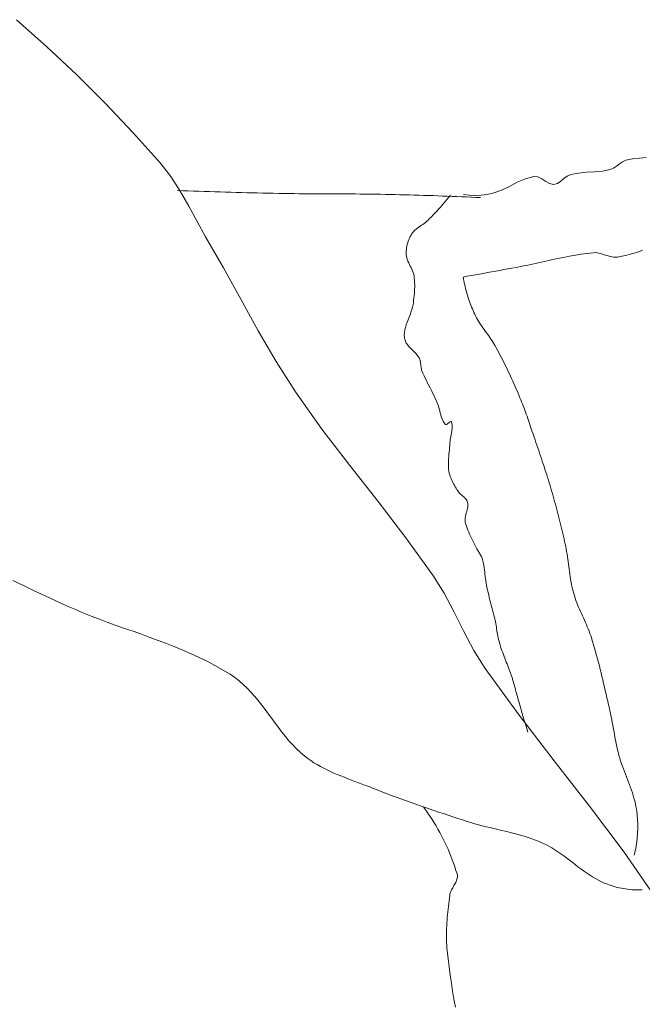
# Model space of a CAD drawing. Units: inches. Extents: x -36302355 to 648, y -221479757 to 75.
# Tile 19 of 37: x 555 to 572, y -501 to -474. Entities that reach past the tile are written whole.
import ezdxf

# ---------------------------------------------------------------- set-up
doc = ezdxf.new("R2010")
doc.units = ezdxf.units.IN
doc.header["$MEASUREMENT"] = 0
doc.layers.add('A-FURN', color=8, linetype='Continuous', lineweight=13)

# ---------------------------------------------------------------- blocks, each defined once
blk = doc.blocks.new('BED-DOUBLE')
for p, q in [((24.695, 63.097), (23.379, 62.192)), ((4.096, 62.613), (4.083, 62.806)), ((6.696, 62.587), (6.657, 62.702)), ((24.428, 62.63), (24.425, 62.688)), ((4.119, 62.421), (4.096, 62.613)), ((4.157, 62.233), (4.119, 62.421)), ((6.733, 62.472), (6.696, 62.587)), ((6.767, 62.356), (6.733, 62.472)), ((21.659, 62.392), (21.585, 62.366)), ((21.733, 62.418), (21.659, 62.392)), ((21.808, 62.442), (21.733, 62.418)), ((21.883, 62.464), (21.808, 62.442)), ((21.958, 62.485), (21.883, 62.464)), ((22.034, 62.503), (21.958, 62.485)), ((22.111, 62.519), (22.034, 62.503)), ((22.188, 62.532), (22.111, 62.519)), ((22.251, 62.541), (22.188, 62.532)), ((22.315, 62.549), (22.251, 62.541)), ((22.378, 62.555), (22.315, 62.549)), ((22.442, 62.561), (22.378, 62.555)), ((22.506, 62.564), (22.442, 62.561)), ((22.57, 62.567), (22.506, 62.564)), ((22.635, 62.568), (22.57, 62.567)), ((22.699, 62.568), (22.635, 62.568)), ((22.763, 62.567), (22.699, 62.568)), ((22.828, 62.565), (22.763, 62.567)), ((22.892, 62.561), (22.828, 62.565)), ((22.956, 62.556), (22.892, 62.561)), ((23.02, 62.55), (22.956, 62.556)), ((23.084, 62.542), (23.02, 62.55)), ((23.148, 62.533), (23.084, 62.542)), ((23.211, 62.523), (23.148, 62.533)), ((23.274, 62.512), (23.211, 62.523)), ((23.337, 62.499), (23.274, 62.512)), ((23.399, 62.485), (23.337, 62.499)), ((23.461, 62.47), (23.399, 62.485)), ((24.417, 62.342), (24.422, 62.4)), ((24.422, 62.4), (24.425, 62.458)), ((24.425, 62.458), (24.428, 62.515)), ((24.428, 62.573), (24.428, 62.63)), ((24.428, 62.515), (24.428, 62.573)), ((4.195, 62.142), (4.157, 62.233)), ((4.253, 62.059), (4.195, 62.142)), ((6.797, 62.24), (6.767, 62.356)), ((6.824, 62.122), (6.797, 62.24)), ((6.846, 62.004), (6.824, 62.122)), ((20.921, 62.115), (20.846, 62.09)), ((20.995, 62.141), (20.921, 62.115)), ((21.069, 62.168), (20.995, 62.141)), ((21.143, 62.196), (21.069, 62.168)), ((21.217, 62.224), (21.143, 62.196)), ((21.29, 62.253), (21.217, 62.224)), ((21.364, 62.282), (21.29, 62.253)), ((21.437, 62.31), (21.364, 62.282)), ((21.511, 62.338), (21.437, 62.31)), ((21.585, 62.366), (21.511, 62.338)), ((23.379, 62.192), (22.102, 61.232)), ((24.371, 62.056), (24.383, 62.113)), ((24.383, 62.113), (24.394, 62.17)), ((24.394, 62.17), (24.403, 62.227)), ((24.403, 62.227), (24.41, 62.285)), ((24.41, 62.285), (24.417, 62.342)), ((4.318, 61.979), (4.253, 62.059)), ((4.377, 61.896), (4.318, 61.979)), ((4.416, 61.805), (4.377, 61.896)), ((6.83, 61.798), (6.842, 61.849)), ((6.842, 61.849), (6.849, 61.9)), ((6.851, 61.952), (6.846, 62.004)), ((6.849, 61.9), (6.851, 61.952)), ((19.645, 61.837), (19.58, 61.824)), ((19.711, 61.849), (19.645, 61.837)), ((19.777, 61.862), (19.711, 61.849)), ((19.843, 61.873), (19.777, 61.862)), ((19.909, 61.885), (19.843, 61.873)), ((19.975, 61.897), (19.909, 61.885)), ((20.041, 61.909), (19.975, 61.897)), ((20.107, 61.92), (20.041, 61.909)), ((20.172, 61.932), (20.107, 61.92)), ((20.238, 61.945), (20.172, 61.932)), ((20.304, 61.957), (20.238, 61.945)), ((20.37, 61.97), (20.304, 61.957)), ((20.435, 61.984), (20.37, 61.97)), ((20.5, 61.998), (20.435, 61.984)), ((20.566, 62.013), (20.5, 61.998)), ((20.631, 62.029), (20.566, 62.013)), ((20.695, 62.046), (20.631, 62.029)), ((20.771, 62.067), (20.695, 62.046)), ((20.846, 62.09), (20.771, 62.067)), ((24.292, 61.778), (24.31, 61.833)), ((24.31, 61.833), (24.327, 61.888)), ((24.327, 61.888), (24.343, 61.944)), ((24.343, 61.944), (24.358, 62)), ((24.358, 62), (24.371, 62.056)), ((4.456, 61.588), (4.416, 61.805)), ((4.476, 61.367), (4.456, 61.588)), ((6.748, 61.541), (6.764, 61.592)), ((6.764, 61.592), (6.781, 61.644)), ((6.781, 61.644), (6.799, 61.695)), ((6.799, 61.695), (6.815, 61.746)), ((6.815, 61.746), (6.83, 61.798)), ((18.498, 61.574), (18.4, 61.551)), ((18.596, 61.598), (18.498, 61.574)), ((18.695, 61.621), (18.596, 61.598)), ((18.793, 61.645), (18.695, 61.621)), ((18.891, 61.667), (18.793, 61.645)), ((18.99, 61.69), (18.891, 61.667)), ((19.088, 61.713), (18.99, 61.69)), ((19.187, 61.736), (19.088, 61.713)), ((19.285, 61.759), (19.187, 61.736)), ((19.383, 61.781), (19.285, 61.759)), ((19.449, 61.796), (19.383, 61.781)), ((19.514, 61.81), (19.449, 61.796)), ((19.58, 61.824), (19.514, 61.81)), ((24.161, 61.478), (24.205, 61.565)), ((24.205, 61.565), (24.228, 61.618)), ((24.228, 61.618), (24.251, 61.67)), ((24.251, 61.67), (24.272, 61.724)), ((24.272, 61.724), (24.292, 61.778)), ((4.49, 61.145), (4.476, 61.367)), ((6.721, 61.386), (6.725, 61.438)), ((6.723, 61.334), (6.721, 61.386)), ((6.742, 61.167), (6.723, 61.334)), ((6.725, 61.438), (6.735, 61.489)), ((6.735, 61.489), (6.748, 61.541)), ((17.426, 61.284), (17.363, 61.264)), ((17.522, 61.314), (17.426, 61.284)), ((17.619, 61.343), (17.522, 61.314)), ((17.716, 61.371), (17.619, 61.343)), ((17.813, 61.398), (17.716, 61.371)), ((17.911, 61.425), (17.813, 61.398)), ((18.008, 61.451), (17.911, 61.425)), ((18.106, 61.477), (18.008, 61.451)), ((18.204, 61.502), (18.106, 61.477)), ((18.302, 61.526), (18.204, 61.502)), ((18.4, 61.551), (18.302, 61.526)), ((24.012, 61.225), (24.064, 61.308)), ((24.064, 61.308), (24.114, 61.392)), ((24.114, 61.392), (24.161, 61.478)), ((4.51, 60.924), (4.49, 61.145)), ((6.765, 61), (6.742, 61.167)), ((16.813, 61.032), (16.752, 61.004)), ((16.873, 61.06), (16.813, 61.032)), ((16.934, 61.087), (16.873, 61.06)), ((16.994, 61.115), (16.934, 61.087)), ((17.055, 61.142), (16.994, 61.115)), ((17.116, 61.168), (17.055, 61.142)), ((17.177, 61.194), (17.116, 61.168)), ((17.238, 61.218), (17.177, 61.194)), ((17.3, 61.242), (17.238, 61.218)), ((17.363, 61.264), (17.3, 61.242)), ((22.102, 61.232), (20.841, 60.248)), ((23.842, 60.984), (23.9, 61.063)), ((23.9, 61.063), (23.957, 61.144)), ((23.957, 61.144), (24.012, 61.225)), ((4.551, 60.707), (4.51, 60.924)), ((6.792, 60.835), (6.765, 61)), ((6.821, 60.669), (6.792, 60.835)), ((15.994, 60.739), (15.926, 60.726)), ((16.062, 60.754), (15.994, 60.739)), ((16.13, 60.771), (16.062, 60.754)), ((16.197, 60.789), (16.13, 60.771)), ((16.261, 60.808), (16.197, 60.789)), ((16.323, 60.828), (16.261, 60.808)), ((16.386, 60.85), (16.323, 60.828)), ((16.448, 60.874), (16.386, 60.85)), ((16.509, 60.898), (16.448, 60.874)), ((16.57, 60.924), (16.509, 60.898)), ((16.631, 60.95), (16.57, 60.924)), ((16.692, 60.977), (16.631, 60.95)), ((16.752, 61.004), (16.692, 60.977)), ((23.602, 60.669), (23.662, 60.748)), ((23.662, 60.748), (23.723, 60.826)), ((23.723, 60.826), (23.783, 60.905)), ((23.783, 60.905), (23.842, 60.984)), ((4.596, 60.607), (4.551, 60.707)), ((4.665, 60.516), (4.596, 60.607)), ((4.738, 60.428), (4.665, 60.516)), ((6.853, 60.504), (6.821, 60.669)), ((6.887, 60.34), (6.853, 60.504)), ((14.45, 60.47), (14.376, 60.452)), ((14.524, 60.487), (14.45, 60.47)), ((14.599, 60.504), (14.524, 60.487)), ((14.673, 60.521), (14.599, 60.504)), ((14.748, 60.538), (14.673, 60.521)), ((14.822, 60.554), (14.748, 60.538)), ((14.891, 60.568), (14.822, 60.554)), ((14.959, 60.581), (14.891, 60.568)), ((15.028, 60.593), (14.959, 60.581)), ((15.097, 60.604), (15.028, 60.593)), ((15.166, 60.614), (15.097, 60.604)), ((15.235, 60.624), (15.166, 60.614)), ((15.304, 60.633), (15.235, 60.624)), ((15.374, 60.642), (15.304, 60.633)), ((15.443, 60.652), (15.374, 60.642)), ((15.512, 60.661), (15.443, 60.652)), ((15.582, 60.67), (15.512, 60.661)), ((15.651, 60.68), (15.582, 60.67)), ((15.72, 60.69), (15.651, 60.68)), ((15.789, 60.701), (15.72, 60.69)), ((15.857, 60.713), (15.789, 60.701)), ((15.926, 60.726), (15.857, 60.713)), ((23.426, 60.431), (23.484, 60.511)), ((23.484, 60.511), (23.542, 60.59)), ((23.542, 60.59), (23.602, 60.669)), ((4.798, 60.335), (4.738, 60.428)), ((4.826, 60.233), (4.798, 60.335)), ((4.805, 60.119), (4.826, 60.233)), ((6.922, 60.175), (6.887, 60.34)), ((13.416, 60.198), (13.343, 60.176)), ((13.489, 60.219), (13.416, 60.198)), ((13.563, 60.239), (13.489, 60.219)), ((13.636, 60.26), (13.563, 60.239)), ((13.71, 60.28), (13.636, 60.26)), ((13.784, 60.3), (13.71, 60.28)), ((13.857, 60.32), (13.784, 60.3)), ((13.931, 60.34), (13.857, 60.32)), ((14.005, 60.359), (13.931, 60.34)), ((14.079, 60.378), (14.005, 60.359)), ((14.153, 60.397), (14.079, 60.378)), ((14.227, 60.416), (14.153, 60.397)), ((14.301, 60.434), (14.227, 60.416)), ((14.376, 60.452), (14.301, 60.434)), ((20.841, 60.248), (19.575, 59.272)), ((23.264, 60.186), (23.316, 60.269)), ((23.316, 60.269), (23.37, 60.351)), ((23.37, 60.351), (23.426, 60.431)), ((4.675, 59.905), (4.746, 60.011)), ((4.746, 60.011), (4.805, 60.119)), ((6.958, 60.011), (6.922, 60.175)), ((6.994, 59.846), (6.958, 60.011)), ((12.519, 59.917), (12.445, 59.892)), ((12.594, 59.942), (12.519, 59.917)), ((12.668, 59.967), (12.594, 59.942)), ((12.743, 59.991), (12.668, 59.967)), ((12.817, 60.015), (12.743, 59.991)), ((12.892, 60.039), (12.817, 60.015)), ((12.967, 60.063), (12.892, 60.039)), ((13.042, 60.086), (12.967, 60.063)), ((13.117, 60.109), (13.042, 60.086)), ((13.192, 60.132), (13.117, 60.109)), ((13.267, 60.154), (13.192, 60.132)), ((13.343, 60.176), (13.267, 60.154)), ((23.085, 59.826), (23.128, 59.926)), ((23.128, 59.926), (23.17, 60.015)), ((23.17, 60.015), (23.215, 60.101)), ((23.215, 60.101), (23.264, 60.186)), ((4.607, 59.685), (4.62, 59.798)), ((4.668, 59.449), (4.607, 59.685)), ((4.62, 59.798), (4.675, 59.905)), ((7.03, 59.682), (6.994, 59.846)), ((7.066, 59.517), (7.03, 59.682)), ((11.734, 59.651), (11.676, 59.631)), ((11.792, 59.671), (11.734, 59.651)), ((11.85, 59.69), (11.792, 59.671)), ((11.924, 59.716), (11.85, 59.69)), ((11.999, 59.741), (11.924, 59.716)), ((12.073, 59.766), (11.999, 59.741)), ((12.147, 59.792), (12.073, 59.766)), ((12.221, 59.817), (12.147, 59.792)), ((12.296, 59.842), (12.221, 59.817)), ((12.37, 59.867), (12.296, 59.842)), ((12.445, 59.892), (12.37, 59.867)), ((23.007, 59.623), (23.045, 59.725)), ((23.045, 59.725), (23.085, 59.826)), ((4.766, 59.224), (4.668, 59.449)), ((7.1, 59.353), (7.066, 59.517)), ((10.924, 59.366), (10.867, 59.344)), ((10.981, 59.388), (10.924, 59.366)), ((11.039, 59.41), (10.981, 59.388)), ((11.096, 59.431), (11.039, 59.41)), ((11.154, 59.452), (11.096, 59.431)), ((11.212, 59.472), (11.154, 59.452)), ((11.269, 59.493), (11.212, 59.472)), ((11.327, 59.513), (11.269, 59.493)), ((11.385, 59.533), (11.327, 59.513)), ((11.443, 59.553), (11.385, 59.533)), ((11.501, 59.572), (11.443, 59.553)), ((11.56, 59.592), (11.501, 59.572)), ((11.618, 59.612), (11.56, 59.592)), ((11.676, 59.631), (11.618, 59.612)), ((19.588, 59.379), (19.523, 59.36)), ((19.653, 59.399), (19.588, 59.379)), ((19.718, 59.418), (19.653, 59.399)), ((19.783, 59.438), (19.718, 59.418)), ((19.848, 59.458), (19.783, 59.438)), ((19.913, 59.478), (19.848, 59.458)), ((19.978, 59.498), (19.913, 59.478)), ((20.043, 59.518), (19.978, 59.498)), ((22.909, 59.313), (22.94, 59.417)), ((22.94, 59.417), (22.973, 59.521)), ((22.973, 59.521), (23.007, 59.623)), ((4.88, 59.003), (4.766, 59.224)), ((7.132, 59.188), (7.1, 59.353)), ((7.153, 59.075), (7.132, 59.188)), ((10.29, 59.097), (10.223, 59.066)), ((10.358, 59.127), (10.29, 59.097)), ((10.425, 59.157), (10.358, 59.127)), ((10.493, 59.187), (10.425, 59.157)), ((10.561, 59.216), (10.493, 59.187)), ((10.629, 59.246), (10.561, 59.216)), ((10.697, 59.275), (10.629, 59.246)), ((10.753, 59.298), (10.697, 59.275)), ((10.81, 59.321), (10.753, 59.298)), ((10.867, 59.344), (10.81, 59.321)), ((19.575, 59.272), (18.281, 58.335)), ((18.58, 59.094), (18.555, 59.086)), ((18.627, 59.108), (18.58, 59.094)), ((18.675, 59.122), (18.627, 59.108)), ((18.722, 59.135), (18.675, 59.122)), ((18.769, 59.149), (18.722, 59.135)), ((18.817, 59.161), (18.769, 59.149)), ((18.864, 59.174), (18.817, 59.161)), ((18.912, 59.187), (18.864, 59.174)), ((18.959, 59.199), (18.912, 59.187)), ((19.007, 59.212), (18.959, 59.199)), ((19.054, 59.225), (19.007, 59.212)), ((19.102, 59.238), (19.054, 59.225)), ((19.149, 59.251), (19.102, 59.238)), ((19.197, 59.264), (19.149, 59.251)), ((19.262, 59.283), (19.197, 59.264)), ((19.327, 59.302), (19.262, 59.283)), ((19.392, 59.321), (19.327, 59.302)), ((19.458, 59.341), (19.392, 59.321)), ((19.523, 59.36), (19.458, 59.341)), ((22.826, 58.996), (22.852, 59.102)), ((22.852, 59.102), (22.88, 59.208)), ((22.88, 59.208), (22.909, 59.313)), ((4.988, 58.78), (4.88, 59.003)), ((7.174, 58.962), (7.153, 59.075)), ((7.195, 58.849), (7.174, 58.962)), ((7.216, 58.737), (7.195, 58.849)), ((9.756, 58.842), (9.69, 58.809)), ((9.822, 58.875), (9.756, 58.842)), ((9.889, 58.908), (9.822, 58.875)), ((9.955, 58.94), (9.889, 58.908)), ((10.022, 58.972), (9.955, 58.94)), ((10.089, 59.004), (10.022, 58.972)), ((10.156, 59.035), (10.089, 59.004)), ((10.223, 59.066), (10.156, 59.035)), ((17.887, 58.837), (17.834, 58.817)), ((17.94, 58.857), (17.887, 58.837)), ((17.993, 58.877), (17.94, 58.857)), ((18.046, 58.898), (17.993, 58.877)), ((18.098, 58.918), (18.046, 58.898)), ((18.151, 58.938), (18.098, 58.918)), ((18.204, 58.958), (18.151, 58.938)), ((18.257, 58.978), (18.204, 58.958)), ((18.282, 58.987), (18.257, 58.978)), ((18.307, 58.996), (18.282, 58.987)), ((18.332, 59.005), (18.307, 58.996)), ((18.356, 59.015), (18.332, 59.005)), ((18.381, 59.024), (18.356, 59.015)), ((18.406, 59.033), (18.381, 59.024)), ((18.431, 59.043), (18.406, 59.033)), ((18.455, 59.052), (18.431, 59.043)), ((18.48, 59.061), (18.455, 59.052)), ((18.505, 59.07), (18.48, 59.061)), ((18.53, 59.078), (18.505, 59.07)), ((18.555, 59.086), (18.53, 59.078)), ((22.775, 58.784), (22.8, 58.89)), ((22.8, 58.89), (22.826, 58.996)), ((5.069, 58.548), (4.988, 58.78)), ((5.103, 58.387), (5.069, 58.548)), ((7.236, 58.624), (7.216, 58.737)), ((7.257, 58.511), (7.236, 58.624)), ((9.22, 58.553), (9.174, 58.522)), ((9.267, 58.582), (9.22, 58.553)), ((9.315, 58.61), (9.267, 58.582)), ((9.363, 58.637), (9.315, 58.61)), ((9.428, 58.672), (9.363, 58.637)), ((9.493, 58.707), (9.428, 58.672)), ((9.559, 58.741), (9.493, 58.707)), ((9.624, 58.776), (9.559, 58.741)), ((9.69, 58.809), (9.624, 58.776)), ((16.723, 58.554), (16.653, 58.536)), ((16.792, 58.571), (16.723, 58.554)), ((16.862, 58.588), (16.792, 58.571)), ((16.933, 58.604), (16.862, 58.588)), ((16.981, 58.615), (16.933, 58.604)), ((17.03, 58.624), (16.981, 58.615)), ((17.079, 58.633), (17.03, 58.624)), ((17.128, 58.642), (17.079, 58.633)), ((17.177, 58.65), (17.128, 58.642)), ((17.226, 58.658), (17.177, 58.65)), ((17.275, 58.666), (17.226, 58.658)), ((17.324, 58.675), (17.275, 58.666)), ((17.372, 58.684), (17.324, 58.675)), ((17.421, 58.693), (17.372, 58.684)), ((17.469, 58.704), (17.421, 58.693)), ((17.518, 58.716), (17.469, 58.704)), ((17.566, 58.728), (17.518, 58.716)), ((17.62, 58.744), (17.566, 58.728)), ((17.674, 58.761), (17.62, 58.744)), ((17.727, 58.779), (17.674, 58.761)), ((17.781, 58.798), (17.727, 58.779)), ((17.834, 58.817), (17.781, 58.798)), ((22.699, 58.465), (22.725, 58.571)), ((22.725, 58.571), (22.75, 58.678)), ((22.75, 58.678), (22.775, 58.784)), ((5.123, 58.222), (5.103, 58.387)), ((7.278, 58.398), (7.257, 58.511)), ((7.298, 58.285), (7.278, 58.398)), ((7.319, 58.172), (7.298, 58.285)), ((8.856, 58.299), (8.81, 58.267)), ((8.901, 58.331), (8.856, 58.299)), ((8.946, 58.364), (8.901, 58.331)), ((8.991, 58.396), (8.946, 58.364)), ((9.037, 58.428), (8.991, 58.396)), ((9.082, 58.46), (9.037, 58.428)), ((9.128, 58.491), (9.082, 58.46)), ((9.174, 58.522), (9.128, 58.491)), ((15.355, 58.28), (15.295, 58.267)), ((15.415, 58.291), (15.355, 58.28)), ((15.476, 58.301), (15.415, 58.291)), ((15.536, 58.31), (15.476, 58.301)), ((15.597, 58.318), (15.536, 58.31)), ((15.658, 58.326), (15.597, 58.318)), ((15.719, 58.333), (15.658, 58.326)), ((15.78, 58.341), (15.719, 58.333)), ((15.841, 58.35), (15.78, 58.341)), ((15.902, 58.359), (15.841, 58.35)), ((15.963, 58.369), (15.902, 58.359)), ((16.023, 58.381), (15.963, 58.369)), ((16.093, 58.396), (16.023, 58.381)), ((16.164, 58.412), (16.093, 58.396)), ((16.234, 58.428), (16.164, 58.412)), ((16.304, 58.446), (16.234, 58.428)), ((16.374, 58.463), (16.304, 58.446)), ((16.443, 58.481), (16.374, 58.463)), ((16.513, 58.5), (16.443, 58.481)), ((16.583, 58.518), (16.513, 58.5)), ((16.653, 58.536), (16.583, 58.518)), ((18.281, 58.335), (17.775, 58.02)), ((22.647, 58.252), (22.674, 58.358)), ((22.674, 58.358), (22.699, 58.465)), ((5.13, 58.056), (5.123, 58.222)), ((5.124, 57.891), (5.13, 58.056)), ((5.181, 57.938), (5.187, 58.07)), ((5.187, 58.07), (5.194, 58.202)), ((7.339, 58.06), (7.319, 58.172)), ((7.36, 57.947), (7.339, 58.06)), ((8.382, 58.018), (8.333, 57.996)), ((8.431, 58.041), (8.382, 58.018)), ((8.481, 58.065), (8.431, 58.041)), ((8.53, 58.09), (8.481, 58.065)), ((8.578, 58.117), (8.53, 58.09)), ((8.626, 58.146), (8.578, 58.117)), ((8.672, 58.175), (8.626, 58.146)), ((8.719, 58.205), (8.672, 58.175)), ((8.765, 58.236), (8.719, 58.205)), ((8.81, 58.267), (8.765, 58.236)), ((14.766, 58.009), (14.711, 57.981)), ((14.82, 58.037), (14.766, 58.009)), ((14.874, 58.064), (14.82, 58.037)), ((14.929, 58.09), (14.874, 58.064)), ((14.953, 58.102), (14.929, 58.09)), ((14.976, 58.115), (14.953, 58.102)), ((15, 58.128), (14.976, 58.115)), ((15.022, 58.143), (15, 58.128)), ((15.045, 58.157), (15.022, 58.143)), ((15.068, 58.171), (15.045, 58.157)), ((15.091, 58.186), (15.068, 58.171)), ((15.114, 58.199), (15.091, 58.186)), ((15.137, 58.213), (15.114, 58.199)), ((15.161, 58.225), (15.137, 58.213)), ((15.185, 58.236), (15.161, 58.225)), ((15.21, 58.245), (15.185, 58.236)), ((15.235, 58.253), (15.21, 58.245)), ((15.295, 58.267), (15.235, 58.253)), ((17.775, 58.02), (17.248, 57.739)), ((22.56, 57.937), (22.59, 58.042)), ((22.59, 58.042), (22.619, 58.147)), ((22.619, 58.147), (22.647, 58.252)), ((5.104, 57.727), (5.124, 57.891)), ((5.17, 57.675), (5.176, 57.807)), ((5.176, 57.807), (5.181, 57.938)), ((7.38, 57.834), (7.36, 57.947)), ((7.4, 57.721), (7.38, 57.834)), ((7.453, 57.73), (7.4, 57.721)), ((7.506, 57.74), (7.453, 57.73)), ((7.559, 57.751), (7.506, 57.74)), ((7.612, 57.762), (7.559, 57.751)), ((7.665, 57.774), (7.612, 57.762)), ((7.718, 57.787), (7.665, 57.774)), ((7.77, 57.801), (7.718, 57.787)), ((7.823, 57.815), (7.77, 57.801)), ((7.875, 57.83), (7.823, 57.815)), ((7.927, 57.846), (7.875, 57.83)), ((7.978, 57.862), (7.927, 57.846)), ((8.03, 57.879), (7.978, 57.862)), ((8.081, 57.897), (8.03, 57.879)), ((8.132, 57.916), (8.081, 57.897)), ((8.183, 57.935), (8.132, 57.916)), ((8.233, 57.955), (8.183, 57.935)), ((8.283, 57.975), (8.233, 57.955)), ((8.333, 57.996), (8.283, 57.975)), ((13.509, 57.734), (13.486, 57.709)), ((13.531, 57.758), (13.509, 57.734)), ((13.554, 57.781), (13.531, 57.758)), ((13.579, 57.801), (13.554, 57.781)), ((13.605, 57.819), (13.579, 57.801)), ((13.633, 57.832), (13.605, 57.819)), ((13.663, 57.842), (13.633, 57.832)), ((13.704, 57.849), (13.663, 57.842)), ((13.746, 57.85), (13.704, 57.849)), ((13.787, 57.847), (13.746, 57.85)), ((13.829, 57.84), (13.787, 57.847)), ((13.871, 57.83), (13.829, 57.84)), ((13.914, 57.819), (13.871, 57.83)), ((13.956, 57.807), (13.914, 57.819)), ((13.998, 57.795), (13.956, 57.807)), ((14.04, 57.785), (13.998, 57.795)), ((14.082, 57.778), (14.04, 57.785)), ((14.124, 57.773), (14.082, 57.778)), ((14.166, 57.773), (14.124, 57.773)), ((14.208, 57.778), (14.166, 57.773)), ((14.266, 57.791), (14.208, 57.778)), ((14.324, 57.808), (14.266, 57.791)), ((14.381, 57.827), (14.324, 57.808)), ((14.437, 57.849), (14.381, 57.827)), ((14.493, 57.873), (14.437, 57.849)), ((14.548, 57.899), (14.493, 57.873)), ((14.603, 57.925), (14.548, 57.899)), ((14.657, 57.953), (14.603, 57.925)), ((14.711, 57.981), (14.657, 57.953)), ((17.248, 57.739), (16.714, 57.469)), ((22.484, 57.701), (22.527, 57.833)), ((22.527, 57.833), (22.56, 57.937)), ((5.159, 57.411), (5.164, 57.543)), ((5.164, 57.543), (5.17, 57.675)), ((13.146, 57.454), (13.106, 57.432)), ((13.186, 57.477), (13.146, 57.454)), ((13.226, 57.5), (13.186, 57.477)), ((13.266, 57.523), (13.226, 57.5)), ((13.305, 57.547), (13.266, 57.523)), ((13.344, 57.571), (13.305, 57.547)), ((13.371, 57.589), (13.344, 57.571)), ((13.396, 57.61), (13.371, 57.589)), ((13.419, 57.633), (13.396, 57.61)), ((13.442, 57.658), (13.419, 57.633)), ((13.464, 57.683), (13.442, 57.658)), ((13.486, 57.709), (13.464, 57.683)), ((16.714, 57.469), (16.186, 57.189)), ((22.398, 57.436), (22.441, 57.568)), ((22.441, 57.568), (22.484, 57.701)), ((23.688, 57.454), (23.59, 57.418)), ((23.786, 57.488), (23.688, 57.454)), ((23.885, 57.52), (23.786, 57.488)), ((23.984, 57.551), (23.885, 57.52)), ((24.014, 57.558), (23.984, 57.551)), ((24.044, 57.56), (24.014, 57.558)), ((24.074, 57.559), (24.044, 57.56)), ((24.103, 57.555), (24.074, 57.559)), ((24.133, 57.548), (24.103, 57.555)), ((24.162, 57.538), (24.133, 57.548)), ((24.191, 57.526), (24.162, 57.538)), ((24.22, 57.513), (24.191, 57.526)), ((24.25, 57.498), (24.22, 57.513)), ((24.279, 57.482), (24.25, 57.498)), ((24.308, 57.465), (24.279, 57.482)), ((24.338, 57.448), (24.308, 57.465)), ((27.467, 57.465), (27.243, 57.428)), ((27.691, 57.503), (27.467, 57.465)), ((5.185, 57.325), (5.129, 57.371)), ((5.149, 57.147), (5.154, 57.279)), ((5.154, 57.279), (5.159, 57.411)), ((5.24, 57.278), (5.185, 57.325)), ((5.295, 57.231), (5.24, 57.278)), ((5.35, 57.183), (5.295, 57.231)), ((5.405, 57.135), (5.35, 57.183)), ((11.451, 57.188), (11.409, 57.165)), ((11.414, 57.394), (11.411, 57.385)), ((11.411, 57.385), (11.414, 57.373)), ((11.425, 57.4), (11.414, 57.394)), ((11.414, 57.373), (11.422, 57.359)), ((11.422, 57.359), (11.433, 57.343)), ((11.469, 57.409), (11.425, 57.4)), ((11.433, 57.343), (11.447, 57.325)), ((11.447, 57.325), (11.461, 57.307)), ((11.491, 57.216), (11.451, 57.188)), ((11.461, 57.307), (11.475, 57.289)), ((11.514, 57.414), (11.469, 57.409)), ((11.475, 57.289), (11.487, 57.271)), ((11.487, 57.271), (11.496, 57.255)), ((11.5, 57.226), (11.491, 57.216)), ((11.496, 57.255), (11.501, 57.239)), ((11.501, 57.239), (11.5, 57.226)), ((11.559, 57.415), (11.514, 57.414)), ((11.604, 57.413), (11.559, 57.415)), ((11.649, 57.409), (11.604, 57.413)), ((11.695, 57.403), (11.649, 57.409)), ((11.741, 57.395), (11.695, 57.403)), ((11.787, 57.386), (11.741, 57.395)), ((11.832, 57.378), (11.787, 57.386)), ((11.878, 57.369), (11.832, 57.378)), ((11.924, 57.362), (11.878, 57.369)), ((11.97, 57.356), (11.924, 57.362)), ((12.015, 57.352), (11.97, 57.356)), ((12.076, 57.348), (12.015, 57.352)), ((12.137, 57.343), (12.076, 57.348)), ((12.198, 57.338), (12.137, 57.343)), ((12.26, 57.331), (12.198, 57.338)), ((12.321, 57.325), (12.26, 57.331)), ((12.382, 57.32), (12.321, 57.325)), ((12.443, 57.315), (12.382, 57.32)), ((12.504, 57.311), (12.443, 57.315)), ((12.565, 57.309), (12.504, 57.311)), ((12.626, 57.309), (12.565, 57.309)), ((12.686, 57.312), (12.626, 57.309)), ((12.747, 57.317), (12.686, 57.312)), ((12.807, 57.325), (12.747, 57.317)), ((12.852, 57.334), (12.807, 57.325)), ((12.895, 57.345), (12.852, 57.334)), ((12.939, 57.359), (12.895, 57.345)), ((12.981, 57.375), (12.939, 57.359)), ((13.023, 57.392), (12.981, 57.375)), ((13.065, 57.412), (13.023, 57.392)), ((13.106, 57.432), (13.065, 57.412)), ((16.186, 57.189), (15.68, 56.875)), ((22.31, 57.171), (22.354, 57.303)), ((22.354, 57.303), (22.398, 57.436)), ((23.11, 57.213), (23.017, 57.167)), ((23.205, 57.258), (23.11, 57.213)), ((23.3, 57.3), (23.205, 57.258)), ((23.396, 57.341), (23.3, 57.3)), ((23.493, 57.381), (23.396, 57.341)), ((23.59, 57.418), (23.493, 57.381)), ((24.367, 57.431), (24.338, 57.448)), ((24.397, 57.415), (24.367, 57.431)), ((24.426, 57.399), (24.397, 57.415)), ((24.456, 57.385), (24.426, 57.399)), ((24.487, 57.372), (24.456, 57.385)), ((24.517, 57.362), (24.487, 57.372)), ((24.548, 57.354), (24.517, 57.362)), ((24.579, 57.348), (24.548, 57.354)), ((24.655, 57.338), (24.579, 57.348)), ((24.732, 57.329), (24.655, 57.338)), ((24.808, 57.32), (24.732, 57.329)), ((24.885, 57.311), (24.808, 57.32)), ((24.962, 57.302), (24.885, 57.311)), ((25.039, 57.294), (24.962, 57.302)), ((25.116, 57.287), (25.039, 57.294)), ((25.193, 57.28), (25.116, 57.287)), ((25.27, 57.274), (25.193, 57.28)), ((25.347, 57.269), (25.27, 57.274)), ((25.424, 57.264), (25.347, 57.269)), ((25.501, 57.261), (25.424, 57.264)), ((25.578, 57.258), (25.501, 57.261)), ((25.655, 57.257), (25.578, 57.258)), ((25.732, 57.257), (25.655, 57.257)), ((25.809, 57.258), (25.732, 57.257)), ((25.886, 57.261), (25.809, 57.258)), ((25.963, 57.265), (25.886, 57.261)), ((26.039, 57.27), (25.963, 57.265)), ((26.116, 57.277), (26.039, 57.27)), ((26.342, 57.302), (26.116, 57.277)), ((26.568, 57.329), (26.342, 57.302)), ((26.793, 57.36), (26.568, 57.329)), ((27.018, 57.393), (26.793, 57.36)), ((27.243, 57.428), (27.018, 57.393)), ((5.139, 56.883), (5.144, 57.015)), ((5.144, 57.015), (5.149, 57.147)), ((5.459, 57.087), (5.405, 57.135)), ((5.513, 57.038), (5.459, 57.087)), ((5.566, 56.989), (5.513, 57.038)), ((5.619, 56.939), (5.566, 56.989)), ((5.671, 56.889), (5.619, 56.939)), ((10.754, 56.937), (10.685, 56.904)), ((10.822, 56.969), (10.754, 56.937)), ((10.892, 56.999), (10.822, 56.969)), ((10.937, 57.017), (10.892, 56.999)), ((10.984, 57.033), (10.937, 57.017)), ((11.032, 57.047), (10.984, 57.033)), ((11.08, 57.06), (11.032, 57.047)), ((11.129, 57.073), (11.08, 57.06)), ((11.177, 57.085), (11.129, 57.073)), ((11.225, 57.098), (11.177, 57.085)), ((11.273, 57.111), (11.225, 57.098)), ((11.319, 57.127), (11.273, 57.111)), ((11.365, 57.144), (11.319, 57.127)), ((11.409, 57.165), (11.365, 57.144)), ((22.177, 56.774), (22.221, 56.906)), ((22.221, 56.906), (22.266, 57.039)), ((22.266, 57.039), (22.31, 57.171)), ((22.561, 56.913), (22.472, 56.858)), ((22.65, 56.967), (22.561, 56.913)), ((22.74, 57.02), (22.65, 56.967)), ((22.831, 57.07), (22.74, 57.02)), ((22.924, 57.12), (22.831, 57.07)), ((23.017, 57.167), (22.924, 57.12)), ((5.131, 56.619), (5.135, 56.751)), ((5.135, 56.751), (5.139, 56.883)), ((5.723, 56.839), (5.671, 56.889)), ((5.775, 56.788), (5.723, 56.839)), ((5.826, 56.736), (5.775, 56.788)), ((5.856, 56.704), (5.826, 56.736)), ((5.885, 56.67), (5.856, 56.704)), ((5.911, 56.634), (5.885, 56.67)), ((5.937, 56.597), (5.911, 56.634)), ((10.142, 56.634), (10.073, 56.604)), ((10.211, 56.666), (10.142, 56.634)), ((10.279, 56.699), (10.211, 56.666)), ((10.347, 56.733), (10.279, 56.699)), ((10.414, 56.767), (10.347, 56.733)), ((10.482, 56.801), (10.414, 56.767)), ((10.55, 56.836), (10.482, 56.801)), ((10.617, 56.87), (10.55, 56.836)), ((10.685, 56.904), (10.617, 56.87)), ((15.68, 56.875), (14.648, 56.132)), ((22.086, 56.511), (22.131, 56.643)), ((22.214, 56.683), (22.13, 56.622)), ((22.131, 56.643), (22.177, 56.774)), ((22.299, 56.743), (22.214, 56.683)), ((22.385, 56.801), (22.299, 56.743)), ((22.472, 56.858), (22.385, 56.801)), ((5.123, 56.355), (5.127, 56.487)), ((5.127, 56.487), (5.131, 56.619)), ((5.962, 56.559), (5.937, 56.597)), ((5.987, 56.522), (5.962, 56.559)), ((6.013, 56.485), (5.987, 56.522)), ((6.039, 56.449), (6.013, 56.485)), ((6.066, 56.414), (6.039, 56.449)), ((6.095, 56.38), (6.066, 56.414)), ((6.125, 56.349), (6.095, 56.38)), ((7.432, 56.362), (7.371, 56.355)), ((7.492, 56.368), (7.432, 56.362)), ((7.553, 56.371), (7.492, 56.368)), ((7.614, 56.373), (7.553, 56.371)), ((7.676, 56.373), (7.614, 56.373)), ((7.737, 56.371), (7.676, 56.373)), ((7.798, 56.369), (7.737, 56.371)), ((7.859, 56.365), (7.798, 56.369)), ((7.92, 56.359), (7.859, 56.365)), ((7.981, 56.353), (7.92, 56.359)), ((9.486, 56.366), (9.445, 56.325)), ((9.528, 56.405), (9.486, 56.366)), ((9.571, 56.442), (9.528, 56.405)), ((9.616, 56.476), (9.571, 56.442)), ((9.663, 56.504), (9.616, 56.476)), ((9.687, 56.515), (9.663, 56.504)), ((9.712, 56.524), (9.687, 56.515)), ((9.738, 56.53), (9.712, 56.524)), ((9.764, 56.535), (9.738, 56.53)), ((9.79, 56.539), (9.764, 56.535)), ((9.817, 56.542), (9.79, 56.539)), ((9.844, 56.545), (9.817, 56.542)), ((9.872, 56.547), (9.844, 56.545)), ((9.899, 56.55), (9.872, 56.547)), ((9.925, 56.554), (9.899, 56.55)), ((9.952, 56.559), (9.925, 56.554)), ((9.977, 56.566), (9.952, 56.559)), ((10.003, 56.574), (9.977, 56.566)), ((10.073, 56.604), (10.003, 56.574)), ((21.993, 56.248), (22.039, 56.379)), ((22.039, 56.379), (22.086, 56.511)), ((5.112, 55.959), (5.115, 56.091)), ((5.115, 56.091), (5.119, 56.223)), ((5.119, 56.223), (5.123, 56.355)), ((6.158, 56.321), (6.125, 56.349)), ((6.194, 56.296), (6.158, 56.321)), ((6.234, 56.272), (6.194, 56.296)), ((6.274, 56.25), (6.234, 56.272)), ((6.317, 56.229), (6.274, 56.25)), ((6.36, 56.211), (6.317, 56.229)), ((6.404, 56.195), (6.36, 56.211)), ((6.449, 56.18), (6.404, 56.195)), ((6.494, 56.168), (6.449, 56.18)), ((6.54, 56.157), (6.494, 56.168)), ((6.586, 56.149), (6.54, 56.157)), ((6.633, 56.143), (6.586, 56.149)), ((6.679, 56.139), (6.633, 56.143)), ((6.725, 56.138), (6.679, 56.139)), ((6.772, 56.139), (6.725, 56.138)), ((6.82, 56.144), (6.772, 56.139)), ((6.867, 56.155), (6.82, 56.144)), ((6.914, 56.169), (6.867, 56.155)), ((6.959, 56.187), (6.914, 56.169)), ((7.005, 56.207), (6.959, 56.187)), ((7.05, 56.229), (7.005, 56.207)), ((7.094, 56.252), (7.05, 56.229)), ((7.139, 56.274), (7.094, 56.252)), ((7.184, 56.296), (7.139, 56.274)), ((7.23, 56.316), (7.184, 56.296)), ((7.276, 56.333), (7.23, 56.316)), ((7.323, 56.346), (7.276, 56.333)), ((7.371, 56.355), (7.323, 56.346)), ((8.042, 56.345), (7.981, 56.353)), ((8.103, 56.337), (8.042, 56.345)), ((8.163, 56.328), (8.103, 56.337)), ((8.235, 56.314), (8.163, 56.328)), ((8.306, 56.294), (8.235, 56.314)), ((8.377, 56.271), (8.306, 56.294)), ((8.448, 56.244), (8.377, 56.271)), ((8.518, 56.217), (8.448, 56.244)), ((8.588, 56.189), (8.518, 56.217)), ((8.658, 56.162), (8.588, 56.189)), ((8.728, 56.137), (8.658, 56.162)), ((8.798, 56.115), (8.728, 56.137)), ((8.869, 56.098), (8.798, 56.115)), ((8.94, 56.087), (8.869, 56.098)), ((9.011, 56.083), (8.94, 56.087)), ((9.084, 56.087), (9.011, 56.083)), ((9.137, 56.097), (9.084, 56.087)), ((9.186, 56.116), (9.137, 56.097)), ((9.233, 56.141), (9.186, 56.116)), ((9.278, 56.171), (9.233, 56.141)), ((9.321, 56.206), (9.278, 56.171)), ((9.363, 56.244), (9.321, 56.206)), ((9.404, 56.284), (9.363, 56.244)), ((9.445, 56.325), (9.404, 56.284)), ((14.648, 56.132), (13.641, 55.355)), ((21.898, 55.986), (21.946, 56.117)), ((21.946, 56.117), (21.993, 56.248)), ((5.106, 55.695), (5.109, 55.827)), ((5.109, 55.827), (5.112, 55.959)), ((21.801, 55.724), (21.85, 55.855)), ((21.85, 55.855), (21.898, 55.986)), ((5.1, 55.422), (5.103, 55.563)), ((5.103, 55.563), (5.106, 55.695)), ((21.701, 55.464), (21.751, 55.594)), ((21.751, 55.594), (21.801, 55.724)), ((5.096, 55.14), (5.098, 55.281)), ((5.098, 55.281), (5.1, 55.422)), ((13.641, 55.355), (12.64, 54.568)), ((21.599, 55.205), (21.65, 55.334)), ((21.65, 55.334), (21.701, 55.464)), ((5.093, 54.857), (5.094, 54.999)), ((5.094, 54.999), (5.096, 55.14)), ((21.486, 54.912), (21.523, 55.01)), ((21.523, 55.01), (21.56, 55.108)), ((21.56, 55.108), (21.599, 55.205)), ((5.091, 54.575), (5.092, 54.716)), ((5.092, 54.716), (5.093, 54.857)), ((21.375, 54.617), (21.412, 54.715)), ((21.412, 54.715), (21.449, 54.814)), ((21.449, 54.814), (21.486, 54.912)), ((5.091, 54.434), (5.091, 54.575)), ((12.64, 54.568), (11.629, 53.795)), ((21.3, 54.42), (21.338, 54.518)), ((21.338, 54.518), (21.375, 54.617)), ((5.09, 54.293), (5.091, 54.434)), ((5.09, 54.152), (5.09, 54.293)), ((21.181, 54.129), (21.222, 54.225)), ((21.222, 54.225), (21.261, 54.323)), ((21.261, 54.323), (21.3, 54.42)), ((5.089, 54.01), (5.09, 54.152)), ((5.089, 53.869), (5.089, 54.01)), ((21.047, 53.846), (21.093, 53.939)), ((21.093, 53.939), (21.138, 54.034)), ((21.138, 54.034), (21.181, 54.129)), ((5.088, 53.728), (5.089, 53.869)), ((5.088, 53.587), (5.088, 53.728)), ((11.629, 53.795), (10.592, 53.06)), ((20.894, 53.576), (20.947, 53.664)), ((20.947, 53.664), (20.998, 53.754)), ((20.998, 53.754), (21.047, 53.846)), ((5.086, 53.304), (5.087, 53.446)), ((5.087, 53.446), (5.088, 53.587)), ((20.714, 53.322), (20.777, 53.405)), ((20.777, 53.405), (20.837, 53.489)), ((20.837, 53.489), (20.894, 53.576)), ((5.083, 53.022), (5.085, 53.163)), ((5.085, 53.163), (5.086, 53.304)), ((20.399, 52.986), (20.509, 53.093)), ((20.509, 53.093), (20.615, 53.205)), ((20.615, 53.205), (20.714, 53.322)), ((5.078, 52.74), (5.081, 52.881)), ((5.081, 52.881), (5.083, 53.022)), ((10.592, 53.06), (9.751, 52.527)), ((20.165, 52.782), (20.284, 52.882)), ((20.284, 52.882), (20.399, 52.986)), ((5.073, 52.445), (5.076, 52.592)), ((5.076, 52.592), (5.078, 52.74)), ((19.794, 52.496), (19.919, 52.59)), ((19.919, 52.59), (20.043, 52.685)), ((20.043, 52.685), (20.165, 52.782)), ((5.066, 52.15), (5.07, 52.297)), ((5.07, 52.297), (5.073, 52.445)), ((9.751, 52.527), (8.89, 52.026)), ((19.416, 52.218), (19.541, 52.311)), ((19.541, 52.311), (19.668, 52.404)), ((19.668, 52.404), (19.794, 52.496)), ((5.059, 51.855), (5.063, 52.002)), ((5.063, 52.002), (5.066, 52.15)), ((8.89, 52.026), (8.018, 51.542)), ((19.05, 51.929), (19.169, 52.027)), ((19.169, 52.027), (19.291, 52.124)), ((19.291, 52.124), (19.416, 52.218)), ((5.052, 51.56), (5.056, 51.708)), ((5.056, 51.708), (5.059, 51.855)), ((18.718, 51.612), (18.824, 51.722)), ((18.824, 51.722), (18.935, 51.827)), ((18.935, 51.827), (19.05, 51.929)), ((5.048, 51.413), (5.052, 51.56)), ((8.018, 51.542), (7.145, 51.061)), ((18.524, 51.377), (18.617, 51.498)), ((18.617, 51.498), (18.718, 51.612)), ((5.04, 51.118), (5.044, 51.265)), ((5.044, 51.265), (5.048, 51.413)), ((18.31, 51.04), (18.438, 51.25)), ((18.438, 51.25), (18.524, 51.377)), ((5.031, 50.823), (5.035, 50.97)), ((5.035, 50.97), (5.04, 51.118)), ((7.145, 51.061), (6.279, 50.567)), ((18.19, 50.826), (18.31, 51.04)), ((5.021, 50.528), (5.026, 50.675)), ((5.026, 50.675), (5.031, 50.823)), ((18.076, 50.609), (18.19, 50.826)), ((5.011, 50.233), (5.016, 50.381)), ((5.016, 50.381), (5.021, 50.528)), ((6.279, 50.567), (5.859, 50.33)), ((17.866, 50.165), (17.968, 50.388)), ((17.968, 50.388), (18.076, 50.609)), ((5.001, 49.938), (5.006, 50.086)), ((5.006, 50.086), (5.011, 50.233)), ((5.434, 50.099), (5.015, 49.86)), ((5.859, 50.33), (5.434, 50.099)), ((17.768, 49.939), (17.866, 50.165)), ((5.015, 49.86), (4.61, 49.601)), ((4.995, 49.791), (5.001, 49.938)), ((17.674, 49.711), (17.768, 49.939)), ((4.61, 49.601), (4.231, 49.307)), ((17.584, 49.482), (17.674, 49.711)), ((4.231, 49.307), (3.391, 48.555)), ((17.411, 49.018), (17.496, 49.25)), ((17.496, 49.25), (17.584, 49.482)), ((17.327, 48.785), (17.411, 49.018)), ((17.244, 48.552), (17.327, 48.785)), ((3.391, 48.555), (2.572, 47.778)), ((17.161, 48.318), (17.244, 48.552)), ((17.078, 48.085), (17.161, 48.318)), ((16.994, 47.852), (17.078, 48.085)), ((2.572, 47.778), (1.775, 46.979)), ((16.819, 47.389), (16.907, 47.62)), ((16.907, 47.62), (16.994, 47.852)), ((16.727, 47.159), (16.819, 47.389)), ((16.632, 46.932), (16.727, 47.159)), ((1.775, 46.979), (1, 46.159)), ((16.532, 46.706), (16.632, 46.932)), ((16.395, 46.407), (16.532, 46.706)), ((16.256, 46.108), (16.395, 46.407)), ((1, 46.159), (0.249, 45.317)), ((16.116, 45.81), (16.256, 46.108)), ((15.975, 45.513), (16.116, 45.81)), ((15.832, 45.216), (15.975, 45.513))]:
    blk.add_line(p, q)

msp = doc.modelspace()

# ---------------------------------------------------------------- block references
at = {"layer": 'A-FURN', "rotation": 270}
msp.add_blockref('BED-DOUBLE', (509.53, -473.482), dxfattribs=at)

doc.saveas('drawing.dxf')
